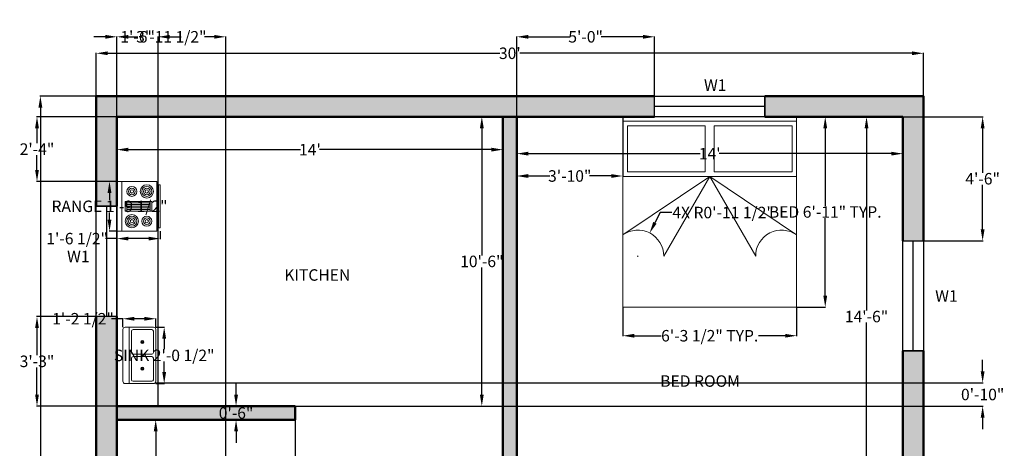
# Model space of a CAD drawing. Units: inches. Extents: x 3136 to 3620, y 13606 to 14152.
# Tile 6 of 6: x 3192 to 3620, y 13965 to 14152. Entities that reach past the tile are written whole.
import ezdxf

# ---------------------------------------------------------------- set-up
doc = ezdxf.new("R2010")
doc.units = ezdxf.units.IN
for name, color, linetype, lineweight in [('A-ANNO-DIMS', 2, 'Continuous', 18), ('A-ANNO-TEXT', 7, 'Continuous', 18), ('A-AREA-IDEN', 7, 'Continuous', 25), ('A-EQPM', 8, 'Continuous', 18), ('A-FLOR-CASE', 8, 'Continuous', 25), ('A-FLOR-FIXT', 9, 'Continuous', 18), ('A-FURN', 8, 'Continuous', 18), ('A-GLAZ', 4, 'Continuous', 25), ('A-WALL', 7, 'Continuous', 50), ('A-WALL-PATT', 174, 'Continuous', 13)]:
    doc.layers.add(name, color=color, linetype=linetype, lineweight=lineweight)
doc.styles.get("Standard").update_dxf_attribs({"font": 'arial.ttf', "height": 5})
doc.dimstyles.get("Standard").update_dxf_attribs({"dimtxt": 5, "dimasz": 5, "dimexe": 0.18, "dimexo": 0.0625, "dimgap": 0.09, "dimtad": 0, "dimtih": 1, "dimtoh": 1, "dimdec": 0, "dimzin": 0, "dimdsep": 46, "dimlunit": 3, "dimtxsty": 'Standard', "dimcen": 0.09, "dimadec": 0, "dimazin": 0, "dimtfac": 1, "dimtdec": 0, "dimtofl": 0, "dimtmove": 0, "dimatfit": 3, "dimfxl": 1, "dimtolj": 1, "dimtzin": 0, "dimarcsym": 0})

# ---------------------------------------------------------------- blocks, each defined once
blk = doc.blocks.new('*D9')
at = {"layer": 'A-ANNO-DIMS', "color": 0, "lineweight": -2, "transparency": 16777216}
for p, q in [((3575.81, 14109.84), (3559.95, 14109.84)), ((3560.13, 14104.84), (3560.13, 14025.48)), ((3560.13, 13940.84), (3560.13, 14020.2)), ((3575.81, 13935.84), (3559.95, 13935.84))]:
    blk.add_line(p, q, dxfattribs=at)
at = {"layer": 'A-ANNO-DIMS', "color": 0, "transparency": 16777216}
for points in [[(3559.29, 14104.84), (3560.96, 14104.84), (3560.13, 14109.84)], [(3559.29, 13940.84), (3560.96, 13940.84), (3560.13, 13935.84)]]:
    blk.add_solid(points, dxfattribs=at)
at = {"layer": 'Defpoints', "color": 0, "transparency": 16777216}
for p in [(3560.13, 14109.84), (3575.87, 14109.84), (3575.87, 13935.84)]:
    blk.add_point(p, dxfattribs=at)
at = {"layer": 'A-ANNO-DIMS', "color": 0, "transparency": 16777216, "insert": (3560.13, 14022.84), "char_height": 5, "attachment_point": 5}
blk.add_mtext('\\A1;14\'-6"', dxfattribs=at)
blk = doc.blocks.new('*D10')
at = {"layer": 'A-ANNO-DIMS', "color": 0, "lineweight": -2, "transparency": 16777216}
for p, q in [((3407.87, 14109.78), (3407.87, 14093.59)), ((3575.87, 14109.78), (3575.87, 14093.59)), ((3412.87, 14093.77), (3487.77, 14093.77)), ((3570.87, 14093.77), (3495.97, 14093.77))]:
    blk.add_line(p, q, dxfattribs=at)
at = {"layer": 'A-ANNO-DIMS', "color": 0, "transparency": 16777216}
for points in [[(3412.87, 14094.6), (3412.87, 14092.94), (3407.87, 14093.77)], [(3570.87, 14094.6), (3570.87, 14092.94), (3575.87, 14093.77)]]:
    blk.add_solid(points, dxfattribs=at)
at = {"layer": 'Defpoints', "color": 0, "transparency": 16777216}
for p in [(3407.87, 14109.84), (3575.87, 14109.84), (3575.87, 14093.77)]:
    blk.add_point(p, dxfattribs=at)
at = {"layer": 'A-ANNO-DIMS', "color": 0, "transparency": 16777216, "insert": (3491.87, 14093.77), "char_height": 5, "attachment_point": 5}
blk.add_mtext("\\A1;14'", dxfattribs=at)
blk = doc.blocks.new('*D11')
at = {"layer": 'A-ANNO-DIMS', "color": 0, "lineweight": -2, "transparency": 16777216}
for p, q in [((3233.87, 14109.78), (3233.87, 14095.33)), ((3401.87, 14109.78), (3401.87, 14095.33)), ((3238.87, 14095.51), (3313.77, 14095.51)), ((3396.87, 14095.51), (3321.97, 14095.51))]:
    blk.add_line(p, q, dxfattribs=at)
at = {"layer": 'A-ANNO-DIMS', "color": 0, "transparency": 16777216}
for points in [[(3238.87, 14096.35), (3238.87, 14094.68), (3233.87, 14095.51)], [(3396.87, 14096.35), (3396.87, 14094.68), (3401.87, 14095.51)]]:
    blk.add_solid(points, dxfattribs=at)
at = {"layer": 'Defpoints', "color": 0, "transparency": 16777216}
for p in [(3233.87, 14109.84), (3401.87, 14109.84), (3401.87, 14095.51)]:
    blk.add_point(p, dxfattribs=at)
at = {"layer": 'A-ANNO-DIMS', "color": 0, "transparency": 16777216, "insert": (3317.87, 14095.51), "char_height": 5, "attachment_point": 5}
blk.add_mtext("\\A1;14'", dxfattribs=at)
blk = doc.blocks.new('*D12')
at = {"layer": 'A-ANNO-DIMS', "color": 0, "lineweight": -2, "transparency": 16777216}
for p, q in [((3379.18, 14109.84), (3392.86, 14109.84)), ((3392.68, 14104.84), (3392.68, 14049.48)), ((3392.68, 13988.84), (3392.68, 14044.2)), ((3379.18, 13983.84), (3392.86, 13983.84))]:
    blk.add_line(p, q, dxfattribs=at)
at = {"layer": 'A-ANNO-DIMS', "color": 0, "transparency": 16777216}
for points in [[(3391.85, 14104.84), (3393.52, 14104.84), (3392.68, 14109.84)], [(3391.85, 13988.84), (3393.52, 13988.84), (3392.68, 13983.84)]]:
    blk.add_solid(points, dxfattribs=at)
at = {"layer": 'Defpoints', "color": 0, "transparency": 16777216}
for p in [(3379.11, 14109.84), (3392.68, 14109.84), (3379.11, 13983.84)]:
    blk.add_point(p, dxfattribs=at)
at = {"layer": 'A-ANNO-DIMS', "color": 0, "transparency": 16777216, "insert": (3392.68, 14046.84), "char_height": 5, "attachment_point": 5}
blk.add_mtext('\\A1;10\'-6"', dxfattribs=at)
blk = doc.blocks.new('*D14')
at = {"layer": 'A-ANNO-DIMS', "color": 0, "lineweight": -2, "transparency": 16777216}
for p, q in [((3233.93, 13977.84), (3250.91, 13977.84)), ((3250.73, 13972.84), (3250.73, 13920.48)), ((3250.73, 13862.84), (3250.73, 13915.2)), ((3233.93, 13857.84), (3250.91, 13857.84))]:
    blk.add_line(p, q, dxfattribs=at)
at = {"layer": 'A-ANNO-DIMS', "color": 0, "transparency": 16777216}
for points in [[(3249.9, 13972.84), (3251.57, 13972.84), (3250.73, 13977.84)], [(3249.9, 13862.84), (3251.57, 13862.84), (3250.73, 13857.84)]]:
    blk.add_solid(points, dxfattribs=at)
at = {"layer": 'Defpoints', "color": 0, "transparency": 16777216}
for p in [(3233.87, 13977.84), (3250.73, 13977.84), (3233.87, 13857.84)]:
    blk.add_point(p, dxfattribs=at)
at = {"layer": 'A-ANNO-DIMS', "color": 0, "transparency": 16777216, "insert": (3250.73, 13917.84), "char_height": 5, "attachment_point": 5}
blk.add_mtext("\\A1;10'", dxfattribs=at)
blk = doc.blocks.new('NEW BED')
for p, q in [((-75.7, 82.92), (0, 82.92)), ((-75.7, 0), (-75.7, 82.92)), ((0, 82.92), (0, 0)), ((-75.7, 80.92), (0, 80.92)), ((-73.7, 78.92), (-39.85, 78.92)), ((-73.7, 58.92), (-73.7, 78.92)), ((-39.85, 58.92), (-39.85, 78.92)), ((-35.85, 78.92), (-2, 78.92)), ((-35.85, 58.92), (-35.85, 78.92)), ((-2, 78.92), (-2, 58.92)), ((-75.7, 56.92), (0, 56.92)), ((-37.85, 56.92), (-75.7, 31.45)), ((-73.7, 58.92), (-39.85, 58.92)), ((-37.85, 56.92), (-57.85, 22.27)), ((-37.85, 56.92), (0, 31.45)), ((-37.85, 56.92), (-17.84, 22.27)), ((-35.85, 58.92), (-2, 58.92)), ((0, 0), (-75.7, 0))]:
    blk.add_line(p, q)
for centre, start, end in [((-69.14, 22.27), 0, 125.5497), ((-6.56, 22.27), 54.4503, 180)]:
    blk.add_arc(centre, 11.28, start, end)
blk = doc.blocks.new('Sink-double - 36 in top')
for p, q in [((-18, -4), (18, -4)), ((-0.75, -18.5), (-0.75, -6.5)), ((0.75, -6.5), (0.75, -18.5))]:
    blk.add_line(p, q)
for points in [[(-16.5, 0), (16.5, 0)], [(-18, -19.5), (-18, -1.5)], [(-15.5, -5.5), (-1.75, -5.5)], [(1.75, -5.5), (15.5, -5.5)], [(18, -1.5), (18, -19.5)], [(-16.5, -18.5), (-16.5, -6.5)], [(16.5, -6.5), (16.5, -18.5)], [(16.5, -21), (-16.5, -21)], [(-1.75, -19.5), (-15.5, -19.5)], [(15.5, -19.5), (1.75, -19.5)]]:
    blk.add_lwpolyline(points)
for centre, radius in [((-8.5, -12.5), 1), ((-8.5, -12.5), 0.5), ((8.5, -12.5), 1), ((8.5, -12.5), 0.5)]:
    blk.add_circle(centre, radius)
for centre, radius, start, end in [((-16.5, -1.5), 1.5, 90, 180), ((16.5, -1.5), 1.5, 0, 90), ((-15.5, -6.5), 1, 90, 180), ((-1.75, -6.5), 1, 0, 90), ((1.75, -6.5), 1, 90, 180), ((15.5, -6.5), 1, 0, 90), ((-15.5, -18.5), 1, 180, 270), ((-1.75, -18.5), 1, 270, 0), ((1.75, -18.5), 1, 180, 270), ((15.5, -18.5), 1, 270, 0), ((-16.5, -19.5), 1.5, 180, 270), ((16.5, -19.5), 1.5, 270, 0)]:
    blk.add_arc(centre, radius, start, end)
blk = doc.blocks.new('Range-Oven - 30 in top')
for p, q in [((0, -3), (30, -3)), ((12, -6), (18, -6)), ((13, -20), (13, -6)), ((14, -6), (14, -20)), ((15, -20), (15, -6)), ((16, -6), (16, -20)), ((17, -20), (17, -6)), ((18, -20), (12, -20)), ((6, -24), (6, -25)), ((8, -25), (8, -24)), ((22, -25), (22, -24)), ((24, -24), (24, -25))]:
    blk.add_line(p, q)
for points in [[(0, -24), (0, 0), (30, 0), (30, -24)], [(12, -21), (12, -5), (18, -5), (18, -21)], [(2, -26), (2, -25), (28, -25), (28, -26)]]:
    blk.add_lwpolyline(points, close=True)
for centre, radius in [((6, -9), 4), ((6, -9), 3), ((6, -9), 2), ((6, -9), 1), ((24, -9), 3), ((24, -9), 2), ((24, -9), 1), ((6, -18), 3), ((6, -18), 2), ((6, -18), 1), ((24, -18), 4), ((24, -18), 3), ((24, -18), 2), ((24, -18), 1)]:
    blk.add_circle(centre, radius)
blk = doc.blocks.new('*D27')
at = {"layer": 'A-ANNO-DIMS', "color": 0, "lineweight": -2, "transparency": 16777216}
for p, q in [((3224.87, 14118.9), (3224.87, 14137.65)), ((3229.87, 14137.47), (3400.54, 14137.47)), ((3579.87, 14137.47), (3409.2, 14137.47)), ((3584.87, 14118.9), (3584.87, 14137.65))]:
    blk.add_line(p, q, dxfattribs=at)
at = {"layer": 'A-ANNO-DIMS', "color": 0, "transparency": 16777216}
for points in [[(3229.87, 14138.31), (3229.87, 14136.64), (3224.87, 14137.47)], [(3579.87, 14138.31), (3579.87, 14136.64), (3584.87, 14137.47)]]:
    blk.add_solid(points, dxfattribs=at)
at = {"layer": 'Defpoints', "color": 0, "transparency": 16777216}
for p in [(3584.87, 14137.47), (3224.87, 14118.84), (3584.87, 14118.84)]:
    blk.add_point(p, dxfattribs=at)
at = {"layer": 'A-ANNO-DIMS', "color": 0, "transparency": 16777216, "insert": (3404.87, 14137.47), "char_height": 5, "attachment_point": 5}
blk.add_mtext("\\A1;30'", dxfattribs=at)
blk = doc.blocks.new('*D28')
at = {"layer": 'A-ANNO-DIMS', "color": 0, "lineweight": -2, "transparency": 16777216}
for p, q in [((3224.81, 14118.84), (3200.37, 14118.84)), ((3200.55, 14113.84), (3200.55, 13881.48)), ((3200.55, 13643.84), (3200.55, 13876.2)), ((3224.81, 13638.84), (3200.37, 13638.84))]:
    blk.add_line(p, q, dxfattribs=at)
at = {"layer": 'A-ANNO-DIMS', "color": 0, "transparency": 16777216}
for points in [[(3199.71, 14113.84), (3201.38, 14113.84), (3200.55, 14118.84)], [(3199.71, 13643.84), (3201.38, 13643.84), (3200.55, 13638.84)]]:
    blk.add_solid(points, dxfattribs=at)
at = {"layer": 'Defpoints', "color": 0, "transparency": 16777216}
for p in [(3200.55, 14118.84), (3224.87, 14118.84), (3224.87, 13638.84)]:
    blk.add_point(p, dxfattribs=at)
at = {"layer": 'A-ANNO-DIMS', "color": 0, "transparency": 16777216, "insert": (3200.55, 13878.84), "char_height": 5, "attachment_point": 5}
blk.add_mtext("\\A1;40'", dxfattribs=at)
blk = doc.blocks.new('WIN-48IN-GLAZING')
for p, q in [((0, 0), (0, 9)), ((48, 0), (48, 9)), ((48, 4.5), (0, 4.5))]:
    blk.add_line(p, q)
blk = doc.blocks.new('*D32')
at = {"layer": 'A-ANNO-DIMS', "color": 0, "lineweight": -2, "transparency": 16777216}
for p, q in [((3529.78, 14109.84), (3542.34, 14109.84)), ((3542.16, 14104.84), (3542.16, 14071.02)), ((3542.16, 14031.92), (3542.16, 14065.74)), ((3529.78, 14026.92), (3542.34, 14026.92))]:
    blk.add_line(p, q, dxfattribs=at)
at = {"layer": 'A-ANNO-DIMS', "color": 0, "transparency": 16777216}
for points in [[(3541.33, 14104.84), (3542.99, 14104.84), (3542.16, 14109.84)], [(3541.33, 14031.92), (3542.99, 14031.92), (3542.16, 14026.92)]]:
    blk.add_solid(points, dxfattribs=at)
at = {"layer": 'Defpoints', "color": 0, "transparency": 16777216}
for p in [(3529.72, 14109.84), (3542.16, 14109.84), (3529.72, 14026.92)]:
    blk.add_point(p, dxfattribs=at)
at = {"layer": 'A-ANNO-DIMS', "color": 0, "transparency": 16777216, "insert": (3542.16, 14068.38), "char_height": 5, "attachment_point": 5}
blk.add_mtext('\\A1;BED 6\'-11" TYP.', dxfattribs=at)
blk = doc.blocks.new('*D33')
at = {"layer": 'A-ANNO-DIMS', "color": 0, "lineweight": -2, "transparency": 16777216}
for p, q in [((3454.02, 14026.86), (3454.02, 14014.3)), ((3529.72, 14026.86), (3529.72, 14014.3)), ((3459.02, 14014.48), (3470.7, 14014.48)), ((3524.72, 14014.48), (3513.04, 14014.48))]:
    blk.add_line(p, q, dxfattribs=at)
at = {"layer": 'A-ANNO-DIMS', "color": 0, "transparency": 16777216}
for points in [[(3459.02, 14015.31), (3459.02, 14013.65), (3454.02, 14014.48)], [(3524.72, 14015.31), (3524.72, 14013.65), (3529.72, 14014.48)]]:
    blk.add_solid(points, dxfattribs=at)
at = {"layer": 'Defpoints', "color": 0, "transparency": 16777216}
for p in [(3454.02, 14026.92), (3529.72, 14026.92), (3529.72, 14014.48)]:
    blk.add_point(p, dxfattribs=at)
at = {"layer": 'A-ANNO-DIMS', "color": 0, "transparency": 16777216, "insert": (3491.87, 14014.48), "char_height": 5, "attachment_point": 5}
blk.add_mtext('\\A1;6\'-3 1/2" TYP.', dxfattribs=at)
blk = doc.blocks.new('*D40')
at = {"layer": 'A-ANNO-DIMS', "color": 0, "lineweight": -2, "transparency": 16777216}
for p, q in [((3250.81, 14018.2), (3254.61, 14018.2)), ((3254.43, 14013.2), (3254.43, 14008.6)), ((3254.43, 13998.65), (3254.43, 14003.25)), ((3250.81, 13993.65), (3254.61, 13993.65))]:
    blk.add_line(p, q, dxfattribs=at)
at = {"layer": 'A-ANNO-DIMS', "color": 0, "transparency": 16777216}
for points in [[(3253.6, 14013.2), (3255.26, 14013.2), (3254.43, 14018.2)], [(3253.6, 13998.65), (3255.26, 13998.65), (3254.43, 13993.65)]]:
    blk.add_solid(points, dxfattribs=at)
at = {"layer": 'Defpoints', "color": 0, "transparency": 16777216}
for p in [(3250.75, 14018.2), (3254.43, 14018.2), (3250.75, 13993.65)]:
    blk.add_point(p, dxfattribs=at)
at = {"layer": 'A-ANNO-DIMS', "color": 0, "transparency": 16777216, "insert": (3254.43, 14005.92), "char_height": 5, "attachment_point": 5}
blk.add_mtext('\\A1;SINK 2\'-0 1/2"', dxfattribs=at)
blk = doc.blocks.new('*D41')
at = {"layer": 'A-ANNO-DIMS', "color": 0, "lineweight": -2, "transparency": 16777216}
for p, q in [((3236.43, 14021.88), (3231.43, 14021.88)), ((3236.43, 14018.26), (3236.43, 14022.06)), ((3245.75, 14021.88), (3241.43, 14021.88)), ((3250.75, 14018.26), (3250.75, 14022.06))]:
    blk.add_line(p, q, dxfattribs=at)
at = {"layer": 'A-ANNO-DIMS', "color": 0, "transparency": 16777216}
for points in [[(3241.43, 14022.71), (3241.43, 14021.04), (3236.43, 14021.88)], [(3245.75, 14022.71), (3245.75, 14021.04), (3250.75, 14021.88)]]:
    blk.add_solid(points, dxfattribs=at)
at = {"layer": 'Defpoints', "color": 0, "transparency": 16777216}
for p in [(3236.43, 14021.88), (3236.43, 14018.2), (3250.75, 14018.2)]:
    blk.add_point(p, dxfattribs=at)
at = {"layer": 'A-ANNO-DIMS', "color": 0, "transparency": 16777216, "insert": (3219.11, 14021.88), "char_height": 5, "attachment_point": 5}
blk.add_mtext('\\A1;1\'-2 1/2"', dxfattribs=at)
blk = doc.blocks.new('*D42')
at = {"layer": 'A-ANNO-DIMS', "color": 0, "lineweight": -2, "transparency": 16777216}
for p, q in [((3233.81, 14081.66), (3230.45, 14081.66)), ((3230.63, 14076.66), (3230.63, 14073.51)), ((3230.63, 14065.02), (3230.63, 14068.16)), ((3233.81, 14060.02), (3230.45, 14060.02))]:
    blk.add_line(p, q, dxfattribs=at)
at = {"layer": 'A-ANNO-DIMS', "color": 0, "transparency": 16777216}
for points in [[(3229.79, 14076.66), (3231.46, 14076.66), (3230.63, 14081.66)], [(3229.79, 14065.02), (3231.46, 14065.02), (3230.63, 14060.02)]]:
    blk.add_solid(points, dxfattribs=at)
at = {"layer": 'Defpoints', "color": 0, "transparency": 16777216}
for p in [(3230.63, 14081.66), (3233.87, 14081.66), (3233.87, 14060.02)]:
    blk.add_point(p, dxfattribs=at)
at = {"layer": 'A-ANNO-DIMS', "color": 0, "transparency": 16777216, "insert": (3230.63, 14070.84), "char_height": 5, "attachment_point": 5}
blk.add_mtext('\\A1;RANGE 1\'-9 1/2"', dxfattribs=at)
blk = doc.blocks.new('*D43')
at = {"layer": 'A-ANNO-DIMS', "color": 0, "lineweight": -2, "transparency": 16777216}
for p, q in [((3233.87, 14059.96), (3233.87, 14056.6)), ((3252.62, 14059.96), (3252.62, 14056.6)), ((3233.87, 14056.78), (3228.87, 14056.78)), ((3247.62, 14056.78), (3238.87, 14056.78))]:
    blk.add_line(p, q, dxfattribs=at)
at = {"layer": 'A-ANNO-DIMS', "color": 0, "transparency": 16777216}
for points in [[(3238.87, 14057.61), (3238.87, 14055.94), (3233.87, 14056.78)], [(3247.62, 14057.61), (3247.62, 14055.94), (3252.62, 14056.78)]]:
    blk.add_solid(points, dxfattribs=at)
at = {"layer": 'Defpoints', "color": 0, "transparency": 16777216}
for p in [(3233.87, 14060.02), (3252.62, 14060.02), (3233.87, 14056.78)]:
    blk.add_point(p, dxfattribs=at)
at = {"layer": 'A-ANNO-DIMS', "color": 0, "transparency": 16777216, "insert": (3216.55, 14056.78), "char_height": 5, "attachment_point": 5}
blk.add_mtext('\\A1;1\'-6 1/2"', dxfattribs=at)
blk = doc.blocks.new('*D54')
at = {"layer": 'A-ANNO-DIMS', "color": 0, "lineweight": -2, "transparency": 16777216}
for p, q in [((3228.87, 14144.64), (3223.87, 14144.64)), ((3233.87, 14109.9), (3233.87, 14144.82)), ((3251.87, 14109.9), (3251.87, 14144.82)), ((3256.87, 14144.64), (3261.87, 14144.64))]:
    blk.add_line(p, q, dxfattribs=at)
at = {"layer": 'A-ANNO-DIMS', "color": 0, "transparency": 16777216}
for points in [[(3228.87, 14145.47), (3228.87, 14143.81), (3233.87, 14144.64)], [(3256.87, 14145.47), (3256.87, 14143.81), (3251.87, 14144.64)]]:
    blk.add_solid(points, dxfattribs=at)
at = {"layer": 'Defpoints', "color": 0, "transparency": 16777216}
for p in [(3251.87, 14144.64), (3233.87, 14109.84), (3251.87, 14109.84)]:
    blk.add_point(p, dxfattribs=at)
at = {"layer": 'A-ANNO-DIMS', "color": 0, "transparency": 16777216, "insert": (3242.87, 14144.64), "char_height": 5, "attachment_point": 5}
blk.add_mtext('\\A1;1\'-6"', dxfattribs=at)
blk = doc.blocks.new('*D55')
at = {"layer": 'A-ANNO-DIMS', "color": 0, "lineweight": -2, "transparency": 16777216}
for p, q in [((3233.87, 13977.78), (3233.87, 13951.86)), ((3311.51, 13977.78), (3311.51, 13951.86)), ((3238.87, 13952.04), (3260.12, 13952.04)), ((3306.51, 13952.04), (3285.27, 13952.04))]:
    blk.add_line(p, q, dxfattribs=at)
at = {"layer": 'A-ANNO-DIMS', "color": 0, "transparency": 16777216}
for points in [[(3238.87, 13952.87), (3238.87, 13951.21), (3233.87, 13952.04)], [(3306.51, 13952.87), (3306.51, 13951.21), (3311.51, 13952.04)]]:
    blk.add_solid(points, dxfattribs=at)
at = {"layer": 'Defpoints', "color": 0, "transparency": 16777216}
for p in [(3233.87, 13977.84), (3311.51, 13977.84), (3233.87, 13952.04)]:
    blk.add_point(p, dxfattribs=at)
at = {"layer": 'A-ANNO-DIMS', "color": 0, "transparency": 16777216, "insert": (3272.69, 13952.04), "char_height": 5, "attachment_point": 5}
blk.add_mtext('\\A1;6\'-5 1/2"', dxfattribs=at)
blk = doc.blocks.new('*D56')
at = {"layer": 'A-ANNO-DIMS', "color": 0, "lineweight": -2, "transparency": 16777216}
for p, q in [((3285.71, 13988.84), (3285.71, 13993.84)), ((3311.45, 13983.84), (3285.53, 13983.84)), ((3311.45, 13977.84), (3285.53, 13977.84)), ((3285.71, 13972.84), (3285.71, 13967.84))]:
    blk.add_line(p, q, dxfattribs=at)
at = {"layer": 'A-ANNO-DIMS', "color": 0, "transparency": 16777216}
for points in [[(3284.88, 13988.84), (3286.55, 13988.84), (3285.71, 13983.84)], [(3284.88, 13972.84), (3286.55, 13972.84), (3285.71, 13977.84)]]:
    blk.add_solid(points, dxfattribs=at)
at = {"layer": 'Defpoints', "color": 0, "transparency": 16777216}
for p in [(3285.71, 13983.84), (3311.51, 13983.84), (3311.51, 13977.84)]:
    blk.add_point(p, dxfattribs=at)
at = {"layer": 'A-ANNO-DIMS', "color": 0, "transparency": 16777216, "insert": (3285.71, 13980.84), "char_height": 5, "attachment_point": 5}
blk.add_mtext('\\A1;0\'-6"', dxfattribs=at)
blk = doc.blocks.new('*D58')
at = {"layer": 'A-ANNO-DIMS', "color": 0, "lineweight": -2, "transparency": 16777216}
for p, q in [((3407.87, 14109.9), (3407.87, 14144.82)), ((3412.87, 14144.64), (3431.14, 14144.64)), ((3462.87, 14144.64), (3444.61, 14144.64)), ((3467.87, 14109.9), (3467.87, 14144.82))]:
    blk.add_line(p, q, dxfattribs=at)
at = {"layer": 'A-ANNO-DIMS', "color": 0, "transparency": 16777216}
for points in [[(3412.87, 14145.47), (3412.87, 14143.81), (3407.87, 14144.64)], [(3462.87, 14145.47), (3462.87, 14143.81), (3467.87, 14144.64)]]:
    blk.add_solid(points, dxfattribs=at)
at = {"layer": 'Defpoints', "color": 0, "transparency": 16777216}
for p in [(3467.87, 14144.64), (3407.87, 14109.84), (3467.87, 14109.84)]:
    blk.add_point(p, dxfattribs=at)
at = {"layer": 'A-ANNO-DIMS', "color": 0, "transparency": 16777216, "insert": (3437.87, 14144.64), "char_height": 5, "attachment_point": 5}
blk.add_mtext('\\A1;5\'-0"', dxfattribs=at)
blk = doc.blocks.new('*D59')
at = {"layer": 'A-ANNO-DIMS', "color": 0, "lineweight": -2, "transparency": 16777216}
for p, q in [((3575.93, 14109.84), (3610.85, 14109.84)), ((3610.67, 14104.84), (3610.67, 14085.48)), ((3610.67, 14060.84), (3610.67, 14080.2)), ((3575.93, 14055.84), (3610.85, 14055.84))]:
    blk.add_line(p, q, dxfattribs=at)
at = {"layer": 'A-ANNO-DIMS', "color": 0, "transparency": 16777216}
for points in [[(3609.84, 14104.84), (3611.5, 14104.84), (3610.67, 14109.84)], [(3609.84, 14060.84), (3611.5, 14060.84), (3610.67, 14055.84)]]:
    blk.add_solid(points, dxfattribs=at)
at = {"layer": 'Defpoints', "color": 0, "transparency": 16777216}
for p in [(3575.87, 14109.84), (3610.67, 14109.84), (3575.87, 14055.84)]:
    blk.add_point(p, dxfattribs=at)
at = {"layer": 'A-ANNO-DIMS', "color": 0, "transparency": 16777216, "insert": (3610.67, 14082.84), "char_height": 5, "attachment_point": 5}
blk.add_mtext('\\A1;4\'-6"', dxfattribs=at)
blk = doc.blocks.new('*D65')
at = {"layer": 'A-ANNO-DIMS', "color": 0, "lineweight": -2, "transparency": 16777216}
for p, q in [((3233.81, 14022.84), (3198.89, 14022.84)), ((3199.07, 14017.84), (3199.07, 14005.98)), ((3199.07, 13988.84), (3199.07, 14000.69)), ((3233.81, 13983.84), (3198.89, 13983.84))]:
    blk.add_line(p, q, dxfattribs=at)
at = {"layer": 'A-ANNO-DIMS', "color": 0, "transparency": 16777216}
for points in [[(3198.24, 14017.84), (3199.9, 14017.84), (3199.07, 14022.84)], [(3198.24, 13988.84), (3199.9, 13988.84), (3199.07, 13983.84)]]:
    blk.add_solid(points, dxfattribs=at)
at = {"layer": 'Defpoints', "color": 0, "transparency": 16777216}
for p in [(3199.07, 14022.84), (3233.87, 14022.84), (3233.87, 13983.84)]:
    blk.add_point(p, dxfattribs=at)
at = {"layer": 'A-ANNO-DIMS', "color": 0, "transparency": 16777216, "insert": (3199.07, 14003.34), "char_height": 5, "attachment_point": 5}
blk.add_mtext('\\A1;3\'-3"', dxfattribs=at)
blk = doc.blocks.new('*D66')
at = {"layer": 'A-ANNO-DIMS', "color": 0, "lineweight": -2, "transparency": 16777216}
for p, q in [((3233.81, 14109.84), (3198.89, 14109.84)), ((3199.07, 14104.84), (3199.07, 14098.35)), ((3199.07, 14086.66), (3199.07, 14093.15)), ((3233.81, 14081.66), (3198.89, 14081.66))]:
    blk.add_line(p, q, dxfattribs=at)
at = {"layer": 'A-ANNO-DIMS', "color": 0, "transparency": 16777216}
for points in [[(3198.24, 14104.84), (3199.9, 14104.84), (3199.07, 14109.84)], [(3198.24, 14086.66), (3199.9, 14086.66), (3199.07, 14081.66)]]:
    blk.add_solid(points, dxfattribs=at)
at = {"layer": 'Defpoints', "color": 0, "transparency": 16777216}
for p in [(3199.07, 14109.84), (3233.87, 14109.84), (3233.87, 14081.66)]:
    blk.add_point(p, dxfattribs=at)
at = {"layer": 'A-ANNO-DIMS', "color": 0, "transparency": 16777216, "insert": (3199.07, 14095.75), "char_height": 5, "attachment_point": 5}
blk.add_mtext('\\A1;2\'-4"', dxfattribs=at)
blk = doc.blocks.new('*D67')
at = {"layer": 'A-ANNO-DIMS', "color": 0, "lineweight": -2, "transparency": 16777216}
for p, q in [((3610.67, 13998.95), (3610.67, 14003.95)), ((3250.51, 13993.95), (3610.85, 13993.95)), ((3251.93, 13983.84), (3610.85, 13983.84)), ((3610.67, 13978.84), (3610.67, 13973.84))]:
    blk.add_line(p, q, dxfattribs=at)
at = {"layer": 'A-ANNO-DIMS', "color": 0, "transparency": 16777216}
for points in [[(3609.84, 13998.95), (3611.5, 13998.95), (3610.67, 13993.95)], [(3609.84, 13978.84), (3611.5, 13978.84), (3610.67, 13983.84)]]:
    blk.add_solid(points, dxfattribs=at)
at = {"layer": 'Defpoints', "color": 0, "transparency": 16777216}
for p in [(3250.45, 13993.95), (3251.87, 13983.84), (3610.67, 13983.84)]:
    blk.add_point(p, dxfattribs=at)
at = {"layer": 'A-ANNO-DIMS', "color": 0, "transparency": 16777216, "insert": (3610.67, 13988.9), "char_height": 5, "attachment_point": 5}
blk.add_mtext('\\A1;0\'-10"', dxfattribs=at)
blk = doc.blocks.new('*D74')
at = {"layer": 'A-ANNO-DIMS', "color": 0, "lineweight": -2, "transparency": 16777216}
for p, q in [((3407.87, 14109.78), (3407.87, 14083.86)), ((3454.02, 14109.78), (3454.02, 14083.86)), ((3412.87, 14084.04), (3422.27, 14084.04)), ((3449.02, 14084.04), (3439.62, 14084.04))]:
    blk.add_line(p, q, dxfattribs=at)
at = {"layer": 'A-ANNO-DIMS', "color": 0, "transparency": 16777216}
for points in [[(3412.87, 14084.87), (3412.87, 14083.21), (3407.87, 14084.04)], [(3449.02, 14084.87), (3449.02, 14083.21), (3454.02, 14084.04)]]:
    blk.add_solid(points, dxfattribs=at)
at = {"layer": 'Defpoints', "color": 0, "transparency": 16777216}
for p in [(3407.87, 14109.84), (3454.02, 14109.84), (3407.87, 14084.04)]:
    blk.add_point(p, dxfattribs=at)
at = {"layer": 'A-ANNO-DIMS', "color": 0, "transparency": 16777216, "insert": (3430.95, 14084.04), "char_height": 5, "attachment_point": 5}
blk.add_mtext('\\A1;3\'-10"', dxfattribs=at)
blk = doc.blocks.new('*D77')
at = {"layer": 'A-ANNO-DIMS', "color": 0, "lineweight": -2, "transparency": 16777216}
for p, q in [((3233.87, 13851.9), (3233.87, 14144.82)), ((3238.87, 14144.64), (3243.03, 14144.64)), ((3276.19, 14144.64), (3272.03, 14144.64)), ((3281.19, 13814.42), (3281.19, 14144.82))]:
    blk.add_line(p, q, dxfattribs=at)
at = {"layer": 'A-ANNO-DIMS', "color": 0, "transparency": 16777216}
for points in [[(3238.87, 14145.47), (3238.87, 14143.81), (3233.87, 14144.64)], [(3276.19, 14145.47), (3276.19, 14143.81), (3281.19, 14144.64)]]:
    blk.add_solid(points, dxfattribs=at)
at = {"layer": 'Defpoints', "color": 0, "transparency": 16777216}
for p in [(3233.87, 14144.64), (3233.87, 13851.84), (3281.19, 13814.36)]:
    blk.add_point(p, dxfattribs=at)
at = {"layer": 'A-ANNO-DIMS', "color": 0, "transparency": 16777216, "insert": (3257.53, 14144.64), "char_height": 5, "attachment_point": 5}
blk.add_mtext('\\A1;3\'-11 1/2"', dxfattribs=at)
blk = doc.blocks.new('*D82')
at = {"layer": 'A-ANNO-DIMS', "color": 0, "lineweight": -2, "transparency": 16777216}
for p, q in [((3470.32, 14068.12), (3468.03, 14063.67)), ((3475.32, 14068.12), (3470.32, 14068.12)), ((3460.49, 14049.19), (3460.67, 14049.19)), ((3460.58, 14049.1), (3460.58, 14049.28))]:
    blk.add_line(p, q, dxfattribs=at)
at = {"layer": 'A-ANNO-DIMS', "color": 0, "transparency": 16777216}
blk.add_solid([(3467.29, 14064.05), (3468.77, 14063.29), (3465.74, 14059.22)], dxfattribs=at)
at = {"layer": 'Defpoints', "color": 0, "transparency": 16777216}
for p in [(3465.74, 14059.22), (3460.58, 14049.19)]:
    blk.add_point(p, dxfattribs=at)
at = {"layer": 'A-ANNO-DIMS', "color": 0, "transparency": 16777216, "insert": (3497.69, 14068.12), "char_height": 5, "attachment_point": 5}
blk.add_mtext('\\A1;4X R0\'-11 1/2"', dxfattribs=at)

msp = doc.modelspace()

# ---------------------------------------------------------------- hatches: boundary and pattern name
at = {"layer": 'A-WALL-PATT'}
h = msp.add_hatch(color=256, dxfattribs=at)
h.dxf.hatch_style = 1
h.paths.add_polyline_path([(3584.87, 13767.84), (3575.87, 13767.84), (3575.87, 13714.7), (3584.87, 13714.7)])
h.paths.add_polyline_path([(3584.87, 13666.7), (3575.87, 13666.7), (3575.87, 13647.84), (3398.03, 13647.84), (3398.03, 13638.84), (3584.87, 13638.84)])
h.paths.add_polyline_path([(3350.03, 13647.84), (3272.91, 13647.84, -0.03225), (3273.24, 13642.78), (3273.24, 13638.84), (3350.03, 13638.84)])
h.paths.add_polyline_path([(3233.87, 13724.63), (3224.87, 13724.63), (3224.87, 13638.84), (3233.87, 13638.84), (3233.87, 13642.78), (3233.87, 13682.15)])
h.paths.add_polyline_path([(3233.87, 13893.84), (3224.87, 13893.84), (3224.87, 13760.63), (3233.87, 13760.63)])
h.paths.add_polyline_path([(3356.82, 13857.84), (3233.87, 13857.84), (3233.87, 13851.84), (3356.82, 13851.84)])
h.paths.add_polyline_path([(3233.87, 14022.84), (3224.87, 14022.84), (3224.87, 13941.84), (3233.87, 13941.84)])
h.paths.add_polyline_path([(3311.51, 13983.84), (3233.87, 13983.84), (3233.87, 13977.84), (3311.51, 13977.84)])
h.paths.add_polyline_path([(3467.87, 14118.84), (3224.87, 14118.84), (3224.87, 14070.84), (3233.87, 14070.84), (3233.87, 14081.66), (3233.87, 14109.84), (3467.87, 14109.84)])
h.paths.add_polyline_path([(3575.87, 13935.84), (3435.35, 13935.84, -0.018734), (3435.43, 13933.78), (3435.43, 13929.84), (3575.87, 13929.84)])
h.paths.add_polyline_path([(3417.35, 13932.93), (3424.89, 13932.93), (3424.89, 13943.24), (3417.35, 13943.24)], flags=9)
h.paths.add_polyline_path([(3561.82, 13786.65), (3573.42, 13786.65), (3573.42, 13796.96), (3561.82, 13796.96)], flags=9)
h.paths.add_polyline_path([(3567.12, 13888.65), (3574.84, 13888.65), (3574.84, 13898.96), (3567.12, 13898.96)], flags=9)
h.paths.add_polyline_path([(3536.01, 13916.38), (3543.73, 13916.38), (3543.73, 13926.69), (3536.01, 13926.69)], flags=9)
h.paths.add_polyline_path([(3509.85, 13733.24), (3521.46, 13733.24), (3521.46, 13743.54), (3509.85, 13743.54)], flags=9)
h.paths.add_polyline_path([(3499.97, 13866.95), (3511.39, 13866.95), (3511.39, 13877.25), (3499.97, 13877.25)], flags=9)
h.paths.add_polyline_path([(3456.03, 13744.65), (3463.57, 13744.65), (3463.57, 13754.96), (3456.03, 13754.96)], flags=9)
h = msp.add_hatch(color=256, dxfattribs=at)
h.dxf.hatch_style = 1
h.paths.add_polyline_path([(3575.87, 13857.84), (3503.87, 13857.84), (3501.81, 13857.84), (3497.87, 13857.84), (3449.87, 13857.84), (3449.87, 13763.84), (3455.87, 13763.84), (3455.87, 13851.84), (3575.87, 13851.84)])
h.paths.add_polyline_path([(3584.87, 13881.84), (3575.87, 13881.84), (3575.87, 13815.84), (3584.87, 13815.84)])
h.paths.add_polyline_path([(3575.87, 13731.84), (3455.87, 13731.84), (3449.87, 13731.84), (3449.87, 13725.84), (3575.87, 13725.84)])
h.paths.add_polyline_path([(3584.87, 14007.84), (3575.87, 14007.84), (3575.87, 13905.84), (3584.87, 13905.84)])
h.paths.add_polyline_path([(3503.87, 13929.84), (3497.87, 13929.84), (3497.87, 13885.4), (3501.81, 13885.4, -0.018734), (3503.87, 13885.32)])
h.paths.add_polyline_path([(3584.87, 14118.84), (3515.87, 14118.84), (3515.87, 14109.84), (3529.72, 14109.84), (3575.87, 14109.84), (3575.87, 14055.84), (3584.87, 14055.84)])
h.paths.add_polyline_path([(3407.87, 14109.84), (3401.87, 14109.84), (3401.87, 13929.84), (3407.87, 13929.84), (3407.87, 13933.78), (3407.87, 13961.34)])

# ---------------------------------------------------------------- linework, layer by layer
at = {"layer": 'A-FLOR-CASE'}
msp.add_line((3251.87, 13983.84), (3251.87, 14109.84), dxfattribs=at)
at = {"layer": 'A-GLAZ'}
for points in [[(3467.87, 14118.84), (3515.87, 14118.84), (3515.87, 14109.84), (3467.87, 14109.84)], [(3224.87, 14070.84), (3233.87, 14070.84), (3233.87, 14022.84), (3224.87, 14022.84)], [(3575.87, 14055.84), (3584.87, 14055.84), (3584.87, 14007.84), (3575.87, 14007.84)]]:
    msp.add_lwpolyline(points, close=True, dxfattribs=at)
at = {"layer": 'A-WALL'}
for p, q in [((3233.87, 14109.84), (3467.87, 14109.84)), ((3233.87, 14070.84), (3233.87, 14109.84)), ((3401.87, 13929.84), (3401.87, 14109.84)), ((3407.87, 13929.84), (3407.87, 14109.84)), ((3515.87, 14109.84), (3575.87, 14109.84)), ((3575.87, 14109.84), (3575.87, 14055.84)), ((3233.87, 13941.84), (3233.87, 14022.84)), ((3575.87, 14007.84), (3575.87, 13905.84)), ((3233.87, 13983.84), (3311.51, 13983.84)), ((3311.51, 13977.84), (3311.51, 13983.84)), ((3233.87, 13977.84), (3311.51, 13977.84))]:
    msp.add_line(p, q, dxfattribs=at)
for points in [[(3224.87, 14070.84), (3224.87, 14118.84), (3467.87, 14118.84)], [(3515.87, 14118.84), (3584.87, 14118.84), (3584.87, 14055.84)], [(3224.87, 13941.84), (3224.87, 14022.84)], [(3584.87, 14007.84), (3584.87, 13905.84)]]:
    msp.add_lwpolyline(points, dxfattribs=at)

# ---------------------------------------------------------------- block references
at = {"layer": 'A-EQPM', "xscale": 0.7211100332127351, "yscale": 0.7211100332127351, "zscale": 0.7211100332127351, "rotation": 90}
msp.add_blockref('Range-Oven - 30 in top', (3233.87, 14060.02), dxfattribs=at)
at = {"layer": 'A-FLOR-FIXT', "xscale": 0.6817939642492598, "yscale": 0.6817939642492598, "zscale": 0.6817939642492598, "rotation": 90}
msp.add_blockref('Sink-double - 36 in top', (3236.43, 14005.92), dxfattribs=at)
at = {"layer": 'A-FURN'}
msp.add_blockref('NEW BED', (3529.72, 14026.92), dxfattribs=at)
at = {"layer": 'A-GLAZ'}
msp.add_blockref('WIN-48IN-GLAZING', (3467.87, 14109.84), dxfattribs=at)
for p, rotation in [((3233.87, 14022.84), 90.00000000000104), ((3575.87, 14055.84), 270.0000000000073)]:
    msp.add_blockref('WIN-48IN-GLAZING', p, dxfattribs=dict(at, rotation=rotation))

# ---------------------------------------------------------------- texts
at = {"layer": 'A-ANNO-TEXT', "char_height": 5, "attachment_point": 1}
for insert in [(3483.14, 14126.11), (3205.92, 14051.49), (3583.78, 14034.29)]:
    msp.add_mtext_dynamic_manual_height_columns('\\pxqc;W1', width=22.2613, gutter_width=25, heights=[0], dxfattribs=dict(at, insert=insert))
at = {"layer": 'A-AREA-IDEN', "char_height": 5, "attachment_point": 1}
for s, width, insert in [('\\pxqc;KITCHEN', 62.4576, (3289.84, 14043.43)), ('BED ROOM ', 39.0633, (3470.33, 13997.25))]:
    msp.add_mtext_dynamic_manual_height_columns(s, width=width, gutter_width=25, heights=[0], dxfattribs=dict(at, insert=insert))

# ---------------------------------------------------------------- dimensions: what is measured, and where the dimension line sits
at = {"layer": 'A-ANNO-DIMS'}
for base, p1, p2, override, picture, middle in [((3233.87, 14144.64), (3281.19, 13814.36), (3233.87, 13851.84), {"dimdec": 1, "dimlfac": 1, "dimrnd": 0, "dimzin": 1, "dimdsep": 46, "dimlunit": 4, "dimfrac": 2}, '*D77', (3257.53, 14144.64)), ((3251.87, 14144.64), (3233.87, 14109.84), (3251.87, 14109.84), {"dimdec": 1, "dimlfac": 1, "dimrnd": 0, "dimzin": 1, "dimdsep": 46, "dimlunit": 4, "dimfrac": 2}, '*D54', (3242.87, 14144.64)), ((3467.87, 14144.64), (3407.87, 14109.84), (3467.87, 14109.84), {"dimdec": 1, "dimlfac": 1, "dimrnd": 0, "dimzin": 1, "dimdsep": 46, "dimlunit": 4, "dimfrac": 2}, '*D58', (3437.87, 14144.64)), ((3584.87, 14137.47), (3224.87, 14118.84), (3584.87, 14118.84), {"dimclrd": 0, "dimclre": 0, "dimclrt": 0}, '*D27', (3404.87, 14137.47)), ((3401.87, 14095.51), (3233.87, 14109.84), (3401.87, 14109.84), {"dimclrd": 0, "dimclre": 0, "dimclrt": 0}, '*D11', (3317.87, 14095.51)), ((3575.87, 14093.77), (3407.87, 14109.84), (3575.87, 14109.84), {"dimclrd": 0, "dimclre": 0, "dimclrt": 0}, '*D10', (3491.87, 14093.77))]:
    dim = msp.add_linear_dim(base=base, p1=p1, p2=p2, dimstyle='Standard', override=override, dxfattribs=at)
    dim.commit()
    dim.dimension.update_dxf_attribs({"geometry": picture, "text_midpoint": middle})
for base, p1, p2, angle, override, picture, middle in [((3200.55, 14118.84), (3224.87, 13638.84), (3224.87, 14118.84), 90, {"dimclrd": 0, "dimclre": 0, "dimclrt": 0}, '*D28', (3200.55, 13878.84)), ((3199.07, 14109.84), (3233.87, 14081.66), (3233.87, 14109.84), 90, {"dimdec": 1, "dimlfac": 1, "dimrnd": 0, "dimzin": 1, "dimdsep": 46, "dimlunit": 4, "dimfrac": 2}, '*D66', (3199.07, 14095.75)), ((3392.68, 14109.84), (3379.11, 13983.84), (3379.11, 14109.84), 90, {"dimclrd": 0, "dimclre": 0, "dimclrt": 0}, '*D12', (3392.68, 14046.84)), ((3407.8713, 14084.0391), (3454.0217, 14109.8391), (3407.8713, 14109.8391), 180, {"dimdec": 1, "dimlfac": 1, "dimrnd": 0, "dimzin": 1, "dimdsep": 46, "dimlunit": 4, "dimfrac": 2}, '*D74', (3430.9465, 14084.0391)), ((3560.13, 14109.84), (3575.87, 13935.84), (3575.87, 14109.84), 90, {"dimclrd": 0, "dimclre": 0, "dimclrt": 0}, '*D9', (3560.13, 14022.84)), ((3610.67, 14109.84), (3575.87, 14055.84), (3575.87, 14109.84), 90, {"dimdec": 1, "dimlfac": 1, "dimrnd": 0, "dimzin": 1, "dimdsep": 46, "dimlunit": 4, "dimfrac": 2}, '*D59', (3610.67, 14082.84)), ((3233.8713, 14056.7775), (3252.6201, 14060.0225), (3233.8713, 14060.0225), 180, {"dimdec": 1, "dimlfac": 1, "dimrnd": 0, "dimzin": 1, "dimdsep": 46, "dimlunit": 4, "dimfrac": 2}, '*D43', (3216.5456, 14056.7775)), ((3236.43, 14021.88), (3250.75, 14018.2), (3236.43, 14018.2), 180, {"dimdec": 1, "dimlfac": 1, "dimrnd": 0, "dimzin": 1, "dimdsep": 46, "dimlunit": 4, "dimfrac": 2}, '*D41', (3219.11, 14021.88)), ((3199.07, 14022.84), (3233.87, 13983.84), (3233.87, 14022.84), 90, {"dimdec": 1, "dimlfac": 1, "dimrnd": 0, "dimzin": 1, "dimdsep": 46, "dimlunit": 4, "dimfrac": 2}, '*D65', (3199.07, 14003.34)), ((3610.67, 13983.84), (3250.45, 13993.95), (3251.87, 13983.84), 90, {"dimdec": 1, "dimlfac": 1, "dimrnd": 0, "dimzin": 1, "dimdsep": 46, "dimlunit": 4, "dimfrac": 2}, '*D67', (3610.67, 13988.9)), ((3285.71, 13983.84), (3311.51, 13977.84), (3311.51, 13983.84), 90, {"dimdec": 1, "dimlfac": 1, "dimrnd": 0, "dimzin": 1, "dimdsep": 46, "dimlunit": 4, "dimfrac": 2}, '*D56', (3285.71, 13980.84)), ((3250.73, 13977.84), (3233.87, 13857.84), (3233.87, 13977.84), 90, {"dimclrd": 0, "dimclre": 0, "dimclrt": 0}, '*D14', (3250.73, 13917.84)), ((3233.87, 13952.04), (3311.51, 13977.84), (3233.87, 13977.84), 180, {"dimdec": 1, "dimlfac": 1, "dimrnd": 0, "dimzin": 1, "dimdsep": 46, "dimlunit": 4, "dimfrac": 2}, '*D55', (3272.69, 13952.04))]:
    dim = msp.add_linear_dim(base=base, p1=p1, p2=p2, angle=angle, dimstyle='Standard', override=override, dxfattribs=at)
    dim.commit()
    dim.dimension.update_dxf_attribs({"geometry": picture, "text_midpoint": middle})
for base, p1, p2, text, picture, middle in [((3542.16, 14109.84), (3529.72, 14026.92), (3529.72, 14109.84), 'BED <> TYP.', '*D32', (3542.16, 14068.38)), ((3230.63, 14081.66), (3233.87, 14060.02), (3233.87, 14081.66), 'RANGE <>', '*D42', (3230.63, 14070.84)), ((3254.4307, 14018.1961), (3250.749, 13993.6515), (3250.749, 14018.1961), 'SINK <>', '*D40', (3254.4307, 14005.9238))]:
    dim = msp.add_linear_dim(base=base, p1=p1, p2=p2, angle=90, text=text, dimstyle='Standard', override={"dimdec": 1, "dimlfac": 1, "dimrnd": 0, "dimzin": 1, "dimdsep": 46, "dimlunit": 4, "dimfrac": 2}, dxfattribs=at)
    dim.commit()
    dim.dimension.update_dxf_attribs({"geometry": picture, "text_midpoint": middle})
dim = msp.add_radius_dim(center=(3460.58, 14049.19), mpoint=(3465.74, 14059.22), text='4X <>', dimstyle='Standard', override={"dimdec": 1, "dimlfac": 1, "dimrnd": 0, "dimzin": 1, "dimdsep": 46, "dimlunit": 4, "dimfrac": 2}, dxfattribs=at)
dim.commit()
dim.dimension.update_dxf_attribs({"geometry": '*D82', "text_midpoint": (3497.69, 14068.12)})
dim = msp.add_linear_dim(base=(3529.72, 14014.48), p1=(3454.02, 14026.92), p2=(3529.72, 14026.92), text='<> TYP.', dimstyle='Standard', override={"dimdec": 1, "dimlfac": 1, "dimrnd": 0, "dimzin": 1, "dimdsep": 46, "dimlunit": 4, "dimfrac": 2}, dxfattribs=at)
dim.commit()
dim.dimension.update_dxf_attribs({"geometry": '*D33', "text_midpoint": (3491.87, 14014.48)})

doc.saveas('drawing.dxf')
